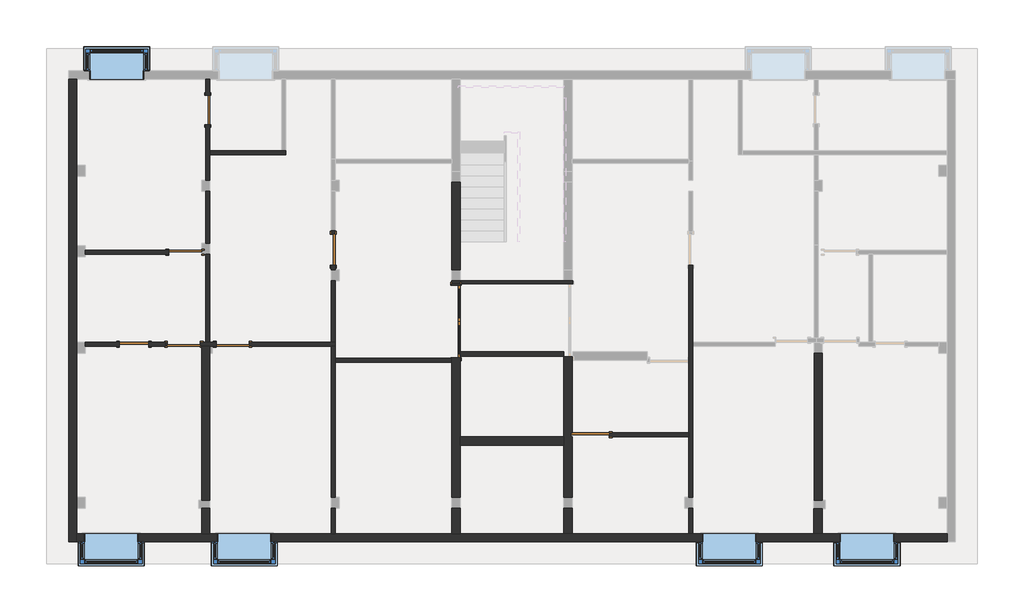
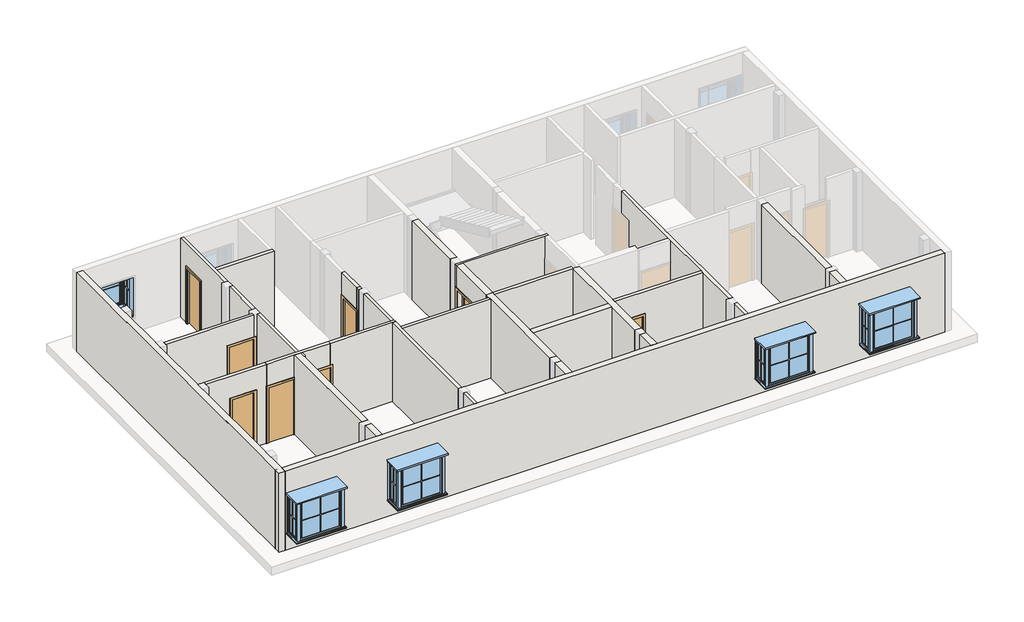
# One storey, part 1 of 3: 33 walls, 8 doors, 5 windows.
"""IFC4 building model written with IfcOpenShell, lengths in millimetres."""

from ifc_helpers import new_model, si_unit, frame, origin, place, context, project, spatial, polyline, outline, extrude, faceted_brep, transform, mapped, element, save
from components import door_77e2dd85, m_door_single_panel_05506f71, door_07b5d71c, door_4c0a2014, door_82def9da, m_door_single_panel_3_x7_f8176753, m_door_single_panel_3_x7_ebb67e73, window_19bbd869

model = new_model("IFC4")

# Units and contexts
model_context = context("Model", 3, world=origin())
ifc_project = project(units=[si_unit("LENGTHUNIT", "METRE", prefix="MILLI")], contexts=[model_context])

# Site, building, storey
site = spatial("IfcSite", under=ifc_project)
building = spatial("IfcBuilding", under=site)
storey = spatial("IfcBuildingStorey", under=building, Elevation=12801.6)

# Doors
placement = place(None, origin())
door_shape = door_77e2dd85(model_context)
element("IfcDoor", 1, ObjectType="M_Door-Double-Glass : 6'7\"X7'", at=placement, inside=storey, context=model_context, shape_type="MappedRepresentation", body=[
    mapped(door_shape, transform((-1965.4800498, 1154.8067742, 12801.6), x_axis=(0.0, -1.0, 0.0), y_axis=(1.0, 0.0, 0.0), z_axis=(0.0, 0.0, 1.0))),
])
m_door_single_panel_shape = m_door_single_panel_05506f71(model_context)
element("IfcDoor", 2, ObjectType="M_Door-Single-Panel", at=placement, inside=storey, context=model_context, shape_type="MappedRepresentation", body=[
    mapped(m_door_single_panel_shape, transform((1745.3012085, -1975.7432663, 12801.6), x_axis=(-1.0, 0.0, 0.0), y_axis=(0.0, -1.0, 0.0), z_axis=(0.0, 0.0, 1.0))),
])
door_2_shape = door_07b5d71c(model_context)
element("IfcDoor", 3, ObjectType="M_Door-Single-Panel : 2'10\"X7' 2", at=placement, inside=storey, context=model_context, shape_type="MappedRepresentation", body=[
    mapped(door_2_shape, transform((-5360.3487995, 3142.9626891, 12801.6), x_axis=(0.0, -1.0, 0.0), y_axis=(1.0, 0.0, 0.0), z_axis=(0.0, 0.0, 1.0))),
])
door_3_shape = door_4c0a2014(model_context)
element("IfcDoor", 4, ObjectType="M_Door-Single-Panel : 2'8\"X7'", at=placement, inside=storey, context=model_context, shape_type="MappedRepresentation", body=[
    mapped(door_3_shape, transform((-10873.4462614, 526.1567334, 12801.6), x_axis=(1.0, 0.0, 0.0), y_axis=(0.0, 1.0, 0.0), z_axis=(0.0, 0.0, 1.0))),
])
door_4_shape = door_82def9da(model_context)
element("IfcDoor", 5, ObjectType="M_Door-Single-Panel : 2'8\"X7'", at=placement, inside=storey, context=model_context, shape_type="MappedRepresentation", body=[
    mapped(door_4_shape, transform((-8827.4487992, 7008.6751452, 12801.6), x_axis=(0.0, 1.0, 0.0), y_axis=(-1.0, 0.0, 0.0), z_axis=(0.0, 0.0, 1.0))),
])
m_door_single_panel_3_x7_shape = m_door_single_panel_3_x7_f8176753(model_context)
element("IfcDoor", 6, ObjectType="M_Door-Single-Panel : 3'X7'", at=placement, inside=storey, context=model_context, shape_type="MappedRepresentation", body=[
    mapped(m_door_single_panel_3_x7_shape, transform((-9456.0987989, 3078.8567332, 12801.6), x_axis=(1.0, 0.0, 0.0), y_axis=(0.0, 1.0, 0.0), z_axis=(0.0, 0.0, 1.0))),
])
element("IfcDoor", 7, ObjectType="M_Door-Single-Panel : 3'X7'", at=placement, inside=storey, context=model_context, shape_type="MappedRepresentation", body=[
    mapped(m_door_single_panel_3_x7_shape, transform((-8144.8381465, 526.1567334, 12801.6), x_axis=(-1.0, 0.0, 0.0), y_axis=(0.0, -1.0, 0.0), z_axis=(0.0, 0.0, 1.0))),
])
m_door_single_panel_3_x7_2_shape = m_door_single_panel_3_x7_ebb67e73(model_context)
element("IfcDoor", 8, ObjectType="M_Door-Single-Panel : 3'X7'", at=placement, inside=storey, context=model_context, shape_type="MappedRepresentation", body=[
    mapped(m_door_single_panel_3_x7_2_shape, transform((-9494.1987992, 526.1567334, 12801.6), x_axis=(1.0, 0.0, 0.0), y_axis=(0.0, 1.0, 0.0), z_axis=(0.0, 0.0, 1.0))),
])

# Walls
element("IfcWall", 9, ObjectType="3.5\"", at=placement, inside=storey, context=model_context, shape_type="Brep", body=[
    faceted_brep([(-2077.3987998, 2196.2067742, 12801.6), (-1848.7987998, 2196.2067742, 12801.6), (1158.0082462, 2196.2067742, 12801.6), (1272.3082462, 2196.2067742, 12801.6), (1272.3082462, 2196.2067742, 15849.6), (1158.0082462, 2196.2067742, 15849.6), (-1848.7987998, 2196.2067742, 15849.6), (-2077.3987998, 2196.2067742, 15849.6), (-2077.3987998, 2285.1067742, 12801.6), (-2077.3987998, 2285.1067742, 15849.6), (-2074.1417538, 2285.1067742, 15849.6), (-1845.5417538, 2285.1067742, 15849.6), (1024.6582462, 2285.1067742, 15849.6), (1253.2582462, 2285.1067742, 15849.6), (1272.3082462, 2285.1067742, 15849.6), (1272.3082462, 2285.1067742, 12801.6), (1253.2582462, 2285.1067742, 12801.6), (1024.6582462, 2285.1067742, 12801.6), (-1845.5417538, 2285.1067742, 12801.6), (-2074.1417538, 2285.1067742, 12801.6)], [[[0, 1, 2, 3, 4, 5, 6, 7]], [[8, 9, 10, 11, 12, 13, 14, 15, 16, 17, 18, 19]], [[3, 2, 1, 0, 8, 19, 18, 17, 16, 15]], [[7, 6, 5, 4, 14, 13, 12, 11, 10, 9]], [[4, 3, 15, 14]], [[0, 7, 9, 8]]]),
])
element("IfcWall", 10, ObjectType="4.5\"", at=placement, inside=storey, context=model_context, shape_type="SweptSolid", body=[
    extrude(outline(polyline([(2711.1626891, 15849.6), (3671.8272228, 15849.6), (3671.8272228, 12801.6), (3574.7626891, 12801.6), (3574.7626891, 14935.2), (2711.1626891, 14935.2), (2711.1626891, 15849.6)])), frame((-5417.4987995, 0.0, 0.0), z_axis=(1.0, 0.0, 0.0), x_axis=(0.0, 1.0, 0.0)), (0.0, 0.0, 1.0), 114.3),
])
element("IfcWall", 11, ObjectType="4.5\"", at=placement, inside=storey, context=model_context, shape_type="Brep", body=[
    faceted_brep([(-7690.1644155, 469.0067334, 15849.6), (-8713.148796, 469.0067334, 15849.6), (-8771.750543, 469.0067334, 15849.6), (-9000.350543, 469.0067334, 15849.6), (-10009.8462614, 469.0067334, 15849.6), (-10009.8462614, 469.0067334, 12801.6), (-9951.3987992, 469.0067334, 12801.6), (-9951.3987992, 469.0067334, 14935.2), (-9036.9987992, 469.0067334, 14935.2), (-9036.9987992, 469.0067334, 12801.6), (-9000.350543, 469.0067334, 12801.6), (-8771.750543, 469.0067334, 12801.6), (-8713.148796, 469.0067334, 12801.6), (-8602.0381465, 469.0067334, 12801.6), (-8602.0381465, 469.0067334, 14935.2), (-7690.1644155, 469.0067334, 14935.2), (-10009.8462614, 583.3067334, 15849.6), (-7690.1644155, 583.3067334, 15849.6), (-7690.1644155, 583.3067334, 14935.2), (-8602.0381465, 583.3067334, 14935.2), (-8602.0381465, 583.3067334, 12801.6), (-9036.9987992, 583.3067334, 12801.6), (-9036.9987992, 583.3067334, 14935.2), (-9951.3987992, 583.3067334, 14935.2), (-9951.3987992, 583.3067334, 12801.6), (-10009.8462614, 583.3067334, 12801.6)], [[[0, 1, 2, 3, 4, 5, 6, 7, 8, 9, 10, 11, 12, 13, 14, 15]], [[16, 17, 18, 19, 20, 21, 22, 23, 24, 25]], [[5, 25, 24, 6]], [[9, 21, 20, 13, 12, 11, 10]], [[17, 0, 15, 18]], [[4, 3, 2, 1, 0, 17, 16]], [[5, 4, 16, 25]], [[8, 22, 21, 9]], [[7, 23, 22, 8]], [[23, 7, 6, 24]], [[19, 14, 13, 20]], [[14, 19, 18, 15]]]),
])
element("IfcWall", 12, ObjectType="4.5\"", at=placement, inside=storey, context=model_context, shape_type="SweptSolid", body=[
    extrude(outline(polyline([(15849.6, 4475.8012082), (15849.6, 1250.0012085), (14935.2, 1250.0012085), (14935.2, 2278.7012085), (12801.6, 2278.7012085), (12801.6, 4475.8012082), (15849.6, 4475.8012082)])), frame((0.0, -2032.8932663, 0.0), z_axis=(0.0, 1.0, 0.0), x_axis=(0.0, 0.0, 1.0)), (0.0, 0.0, 1.0), 114.3),
])
element("IfcWall", 13, ObjectType="4.5\"", at=placement, inside=storey, context=model_context, shape_type="Brep", body=[
    faceted_brep([(-1848.7987998, 202.3067742, 12801.6), (1021.4012085, 202.3067742, 12801.6), (1021.4012085, 202.3067742, 15849.6), (-1848.7987998, 202.3067742, 15849.6), (-1848.7987998, 316.6067742, 12801.6), (-1848.7987998, 316.6067742, 14935.2), (-1848.7987998, 316.6067742, 15849.6), (1021.4012085, 316.6067742, 15849.6), (1021.4012085, 316.6067742, 12801.6)], [[[0, 1, 2, 3]], [[4, 5, 6, 7, 8]], [[1, 0, 4, 8]], [[2, 1, 8, 7]], [[3, 2, 7, 6]], [[0, 3, 6, 5, 4]]]),
])
element("IfcWall", 14, ObjectType="4.5\"", at=placement, inside=storey, context=model_context, shape_type="Brep", body=[
    faceted_brep([(-5417.4987995, 469.0067334, 12801.6), (-5417.4987995, -3709.2932193, 12801.6), (-5417.4987995, -3709.2932193, 15849.6), (-5417.4987995, 469.0067334, 15849.6), (-5303.1987995, 469.0067334, 12801.6), (-5303.1987995, 469.0067334, 15849.6), (-5303.1987995, 148.1078621, 15849.6), (-5303.1987995, 33.8078621, 15849.6), (-5303.1987995, -3709.2932193, 15849.6), (-5303.1987995, -3709.2932193, 12801.6), (-5303.1987995, 33.8078621, 12801.6), (-5303.1987995, 148.1078621, 12801.6)], [[[0, 1, 2, 3]], [[4, 5, 6, 7, 8, 9, 10, 11]], [[1, 0, 4, 11, 10, 9]], [[2, 1, 9, 8]], [[3, 2, 8, 7, 6, 5]], [[0, 3, 5, 4]]]),
])
element("IfcWall", 15, ObjectType="4.5\"", at=placement, inside=storey, context=model_context, shape_type="SweptSolid", body=[
    extrude(outline(polyline([(-5417.4987963, -4712.5932661), (-5417.4987963, -4014.0932193), (-5303.1987963, -4014.0932193), (-5303.1987963, -4712.5932661), (-5417.4987963, -4712.5932661)])), frame((0.0, 0.0, 12801.6), z_axis=(0.0, 0.0, 1.0), x_axis=(1.0, 0.0, 0.0)), (0.0, 0.0, 1.0), 3048.0),
])
element("IfcWall", 16, ObjectType="4.5\"", at=placement, inside=storey, context=model_context, shape_type="SweptSolid", body=[
    extrude(outline(polyline([(4475.8012082, -4712.5932661), (4475.8012082, -4014.0932193), (4590.1012082, -4014.0932193), (4590.1012082, -4712.5932661), (4475.8012082, -4712.5932661)])), frame((0.0, 0.0, 12801.6), z_axis=(0.0, 0.0, 1.0), x_axis=(1.0, 0.0, 0.0)), (0.0, 0.0, 1.0), 3048.0),
])
element("IfcWall", 17, ObjectType="4.5\" 2", at=placement, inside=storey, context=model_context, shape_type="SweptSolid", body=[
    extrude(outline(polyline([(15849.6, -8998.8987989), (15849.6, -12224.6987989), (12801.6, -12224.6987989), (12801.6, -9913.2987989), (14935.2, -9913.2987989), (14935.2, -8998.8987989), (15849.6, -8998.8987989)])), frame((0.0, 3021.7067332, 0.0), z_axis=(0.0, 1.0, 0.0), x_axis=(0.0, 0.0, 1.0)), (0.0, 0.0, 1.0), 114.3),
])
element("IfcWall", 18, ObjectType="4.5\" 2", at=placement, inside=storey, context=model_context, shape_type="SweptSolid", body=[
    extrude(outline(polyline([(-8770.2987992, 4761.606733), (-8770.2987992, 3326.5067332), (-8884.5987992, 3326.5067332), (-8884.5987992, 4761.606733), (-8770.2987992, 4761.606733)])), frame((0.0, 0.0, 12801.6), z_axis=(0.0, 0.0, 1.0), x_axis=(1.0, 0.0, 0.0)), (0.0, 0.0, 1.0), 3048.0),
])
element("IfcWall", 19, ObjectType="4.5\" 2", at=placement, inside=storey, context=model_context, shape_type="Brep", body=[
    faceted_brep([(-8770.2987992, 7415.0751452, 14935.2), (-8770.2987992, 7415.0751452, 12801.6), (-8770.2987992, 7860.4067329, 12801.6), (-8770.2987992, 7860.4067329, 15849.6), (-8770.2987992, 5879.2067329, 15849.6), (-8770.2987992, 5764.9067329, 15849.6), (-8770.2987992, 5066.406733, 15849.6), (-8770.2987992, 5066.406733, 12801.6), (-8770.2987992, 5764.9067329, 12801.6), (-8770.2987992, 5879.2067329, 12801.6), (-8770.2987992, 6602.2751452, 12801.6), (-8770.2987992, 6602.2751452, 14935.2), (-8884.5987992, 7860.4067329, 12801.6), (-8884.5987992, 7415.0751452, 12801.6), (-8884.5987992, 7415.0751452, 14935.2), (-8884.5987992, 6602.2751452, 14935.2), (-8884.5987992, 6602.2751452, 12801.6), (-8884.5987992, 5066.406733, 12801.6), (-8884.5987992, 5066.406733, 15849.6), (-8884.5987992, 7860.4067329, 15849.6)], [[[0, 1, 2, 3, 4, 5, 6, 7, 8, 9, 10, 11]], [[12, 13, 14, 15, 16, 17, 18, 19]], [[2, 1, 13, 12]], [[10, 9, 8, 7, 17, 16]], [[6, 5, 4, 3, 19, 18]], [[7, 6, 18, 17]], [[14, 13, 1, 0]], [[15, 14, 0, 11]], [[16, 15, 11, 10]], [[3, 2, 12, 19]]]),
])
element("IfcWall", 20, ObjectType="4.5\" 2", at=placement, inside=storey, context=model_context, shape_type="Brep", body=[
    faceted_brep([(-8770.2987992, 5764.9067329, 12801.6), (-6674.7987994, 5764.9067329, 12801.6), (-6674.7987994, 5764.9067329, 15849.6), (-8770.2987992, 5764.9067329, 15849.6), (-8770.2987992, 5879.2067329, 12801.6), (-8770.2987992, 5879.2067329, 15849.6), (-6789.0987994, 5879.2067329, 15849.6), (-6674.7987994, 5879.2067329, 15849.6), (-6674.7987994, 5879.2067329, 12801.6), (-6789.0987994, 5879.2067329, 12801.6)], [[[0, 1, 2, 3]], [[4, 5, 6, 7, 8, 9]], [[1, 0, 4, 9, 8]], [[3, 2, 7, 6, 5]], [[0, 3, 5, 4]], [[2, 1, 8, 7]]]),
])
element("IfcWall", 21, ObjectType="4.5\" 2", at=placement, inside=storey, context=model_context, shape_type="SweptSolid", body=[
    extrude(outline(polyline([(14935.2, -10467.0462614), (12801.6, -10467.0462614), (12801.6, -10009.8462614), (15849.6, -10009.8462614), (15849.6, -12224.6987989), (12801.6, -12224.6987989), (12801.6, -11279.8462614), (14935.2, -11279.8462614), (14935.2, -10467.0462614)])), frame((0.0, 469.0067334, 0.0), z_axis=(0.0, 1.0, 0.0), x_axis=(0.0, 0.0, 1.0)), (0.0, 0.0, 1.0), 114.3),
])
element("IfcWall", 22, ObjectType="4.5\" 2", at=placement, inside=storey, context=model_context, shape_type="SweptSolid", body=[
    extrude(outline(polyline([(-8770.298796, 3021.7067332), (-8770.298796, 583.3067804), (-8884.598796, 583.3067804), (-8884.598796, 3021.7067332), (-8770.298796, 3021.7067332)])), frame((0.0, 0.0, 12801.6), z_axis=(0.0, 0.0, 1.0), x_axis=(1.0, 0.0, 0.0)), (0.0, 0.0, 1.0), 3048.0),
])
element("IfcWall", 23, ObjectType="4.5\" 2", at=placement, inside=storey, context=model_context, shape_type="Brep", body=[
    faceted_brep([(-5303.1987995, 469.0067334, 15849.6), (-5417.4987995, 469.0067334, 15849.6), (-7690.1644155, 469.0067334, 15849.6), (-7690.1644155, 469.0067334, 14935.2), (-7687.6381465, 469.0067334, 14935.2), (-7687.6381465, 469.0067334, 12801.6), (-5417.4987995, 469.0067334, 12801.6), (-5303.1987995, 469.0067334, 12801.6), (-7690.1644155, 583.3067334, 15849.6), (-5417.4987995, 583.3067334, 15849.6), (-5303.1987995, 583.3067334, 15849.6), (-5303.1987995, 583.3067334, 12801.6), (-5417.4987995, 583.3067334, 12801.6), (-7687.6381465, 583.3067334, 12801.6), (-7687.6381465, 583.3067334, 14935.2), (-7690.1644155, 583.3067334, 14935.2)], [[[0, 1, 2, 3, 4, 5, 6, 7]], [[8, 9, 10, 11, 12, 13, 14, 15]], [[11, 7, 6, 5, 13, 12]], [[2, 1, 0, 10, 9, 8]], [[2, 8, 15, 3]], [[0, 7, 11, 10]], [[14, 4, 3, 15]], [[4, 14, 13, 5]]]),
])
element("IfcWall", 24, ObjectType="4.5\" 2", at=placement, inside=storey, context=model_context, shape_type="SweptSolid", body=[
    extrude(outline(polyline([(-5303.1987995, 2285.1067802), (-5303.1987995, 583.3067334), (-5417.4987995, 583.3067334), (-5417.4987995, 2285.1067802), (-5303.1987995, 2285.1067802)])), frame((0.0, 0.0, 12801.6), z_axis=(0.0, 0.0, 1.0), x_axis=(1.0, 0.0, 0.0)), (0.0, 0.0, 1.0), 3048.0),
])
element("IfcWall", 25, ObjectType="4.5\" 2", at=placement, inside=storey, context=model_context, shape_type="Brep", body=[
    faceted_brep([(-5303.1987995, 2589.9067802, 12801.6), (-5303.1987995, 2711.1626891, 12801.6), (-5303.1987995, 2711.1626891, 14935.2), (-5303.1987995, 2711.1626891, 15849.6), (-5303.1987995, 2589.9067802, 15849.6), (-5417.4987995, 2589.9067802, 12801.6), (-5417.4987995, 2589.9067802, 15849.6), (-5417.4987995, 2711.1626891, 15849.6), (-5417.4987995, 2711.1626891, 14935.2), (-5417.4987995, 2711.1626891, 12801.6)], [[[0, 1, 2, 3, 4]], [[5, 6, 7, 8, 9]], [[1, 0, 5, 9]], [[3, 2, 1, 9, 8, 7]], [[4, 3, 7, 6]], [[0, 4, 6, 5]]]),
])
element("IfcWall", 26, ObjectType="4.5\" 2", at=placement, inside=storey, context=model_context, shape_type="Brep", body=[
    faceted_brep([(4475.8012082, -3709.2932193, 12801.6), (4475.8012082, -3709.2932193, 15849.6), (4475.8012082, -2032.8932663, 15849.6), (4475.8012082, -1918.5932663, 15849.6), (4475.8012082, 33.8078621, 15849.6), (4475.8012082, 148.1078621, 15849.6), (4475.8012082, 3132.0737955, 15849.6), (4475.8012082, 3132.0737955, 14935.2), (4475.8012082, 2711.1626891, 14935.2), (4475.8012082, 2711.1626891, 12801.6), (4475.8012082, 148.1078621, 12801.6), (4475.8012082, 33.8078621, 12801.6), (4475.8012082, -1918.5932663, 12801.6), (4475.8012082, -2032.8932663, 12801.6), (4590.1012082, -3709.2932193, 15849.6), (4590.1012082, -3709.2932193, 12801.6), (4590.1012082, 469.0067334, 12801.6), (4590.1012082, 583.3067334, 12801.6), (4590.1012082, 2711.1626891, 12801.6), (4590.1012082, 2711.1626891, 14935.2), (4590.1012082, 3132.0737955, 14935.2), (4590.1012082, 3132.0737955, 15849.6), (4590.1012082, 583.3067334, 15849.6), (4590.1012082, 469.0067334, 15849.6)], [[[0, 1, 2, 3, 4, 5, 6, 7, 8, 9, 10, 11, 12, 13]], [[14, 15, 16, 17, 18, 19, 20, 21, 22, 23]], [[15, 0, 13, 12, 11, 10, 9, 18, 17, 16]], [[1, 0, 15, 14]], [[6, 5, 4, 3, 2, 1, 14, 23, 22, 21]], [[6, 21, 20, 7]], [[8, 19, 18, 9]], [[19, 8, 7, 20]]]),
])
element("IfcWall", 27, ObjectType="4.5\" 2", at=placement, inside=storey, context=model_context, shape_type="SweptSolid", body=[
    extrude(outline(polyline([(-2077.3987998, 33.8078621), (-5303.1987995, 33.8078621), (-5303.1987995, 148.1078621), (-2077.3987998, 148.1078621), (-2077.3987998, 33.8078621)])), frame((0.0, 0.0, 12801.6), z_axis=(0.0, 0.0, 1.0), x_axis=(1.0, 0.0, 0.0)), (0.0, 0.0, 1.0), 3048.0),
])
element("IfcWall", 28, ObjectType="9\"", at=placement, inside=storey, context=model_context, shape_type="Brep", body=[
    faceted_brep([(-12453.2987957, -4941.1932661, 12801.6), (-12453.2987957, -4712.5932661, 12801.6), (-12453.2987957, -4014.0932671, 12801.6), (-12453.2987957, -3709.2932671, 12801.6), (-12453.2987957, 278.5067334, 12801.6), (-12453.2987957, 583.3067334, 12801.6), (-12453.2987957, 2951.8567332, 12801.6), (-12453.2987957, 3256.6567332, 12801.6), (-12453.2987957, 5174.3567339, 12801.6), (-12453.2987957, 5479.1567339, 12801.6), (-12453.2987957, 7860.4067329, 12801.6), (-12453.2987957, 7860.4067329, 15849.6), (-12453.2987957, 5479.1567339, 15849.6), (-12453.2987957, 5174.3567339, 15849.6), (-12453.2987957, 3256.6567332, 15849.6), (-12453.2987957, 2951.8567332, 15849.6), (-12453.2987957, 583.3067334, 15849.6), (-12453.2987957, 278.5067334, 15849.6), (-12453.2987957, -3709.2932671, 15849.6), (-12453.2987957, -4014.0932671, 15849.6), (-12453.2987957, -4712.5932661, 15849.6), (-12453.2987957, -4941.1932661, 15849.6), (-12681.8987957, -4941.1932661, 12801.6), (-12681.8987957, -4941.1932661, 15849.6), (-12681.8987957, 7860.4067329, 15849.6), (-12681.8987957, 7860.4067329, 12801.6)], [[[0, 1, 2, 3, 4, 5, 6, 7, 8, 9, 10, 11, 12, 13, 14, 15, 16, 17, 18, 19, 20, 21]], [[22, 23, 24, 25]], [[10, 9, 8, 7, 6, 5, 4, 3, 2, 1, 0, 22, 25]], [[21, 20, 19, 18, 17, 16, 15, 14, 13, 12, 11, 24, 23]], [[11, 10, 25, 24]], [[0, 21, 23, 22]]]),
])
element("IfcWall", 29, ObjectType="9\"", at=placement, inside=storey, context=model_context, shape_type="Brep", body=[
    faceted_brep([(-12453.2987957, -4712.5932661, 12801.6), (-12453.2987957, -4014.0932671, 12801.6), (-12453.2987957, -3709.2932671, 12801.6), (-12453.2987957, 278.5067334, 12801.6), (-12453.2987957, 583.3067334, 12801.6), (-12453.2987957, 2951.8567332, 12801.6), (-12453.2987957, 3256.6567332, 12801.6), (-12453.2987957, 5174.3567339, 12801.6), (-12453.2987957, 5479.1567339, 12801.6), (-12453.2987957, 7860.4067329, 12801.6), (-12453.2987957, 7860.4067329, 15849.6), (-12453.2987957, 5479.1567339, 15849.6), (-12453.2987957, 5174.3567339, 15849.6), (-12453.2987957, 3256.6567332, 15849.6), (-12453.2987957, 2951.8567332, 15849.6), (-12453.2987957, 583.3067334, 15849.6), (-12453.2987957, 278.5067334, 15849.6), (-12453.2987957, -3709.2932671, 15849.6), (-12453.2987957, -4014.0932671, 15849.6), (-12453.2987957, -4712.5932661, 15849.6), (-12681.8987957, -4712.5932661, 12801.6), (-12681.8987957, -4712.5932661, 15849.6), (-12681.8987957, 7860.4067329, 15849.6), (-12681.8987957, 7860.4067329, 12801.6)], [[[0, 1, 2, 3, 4, 5, 6, 7, 8, 9, 10, 11, 12, 13, 14, 15, 16, 17, 18, 19]], [[20, 21, 22, 23]], [[9, 8, 7, 6, 5, 4, 3, 2, 1, 0, 20, 23]], [[19, 18, 17, 16, 15, 14, 13, 12, 11, 10, 22, 21]], [[10, 9, 23, 22]], [[0, 19, 21, 20]]]),
])
element("IfcWall", 30, ObjectType="9\"", at=placement, inside=storey, context=model_context, shape_type="Brep", body=[
    faceted_brep([(-9000.350543, 469.0067334, 12801.6), (-9000.350543, -3785.4932196, 12801.6), (-9000.350543, -3785.4932196, 15849.6), (-9000.350543, 469.0067334, 15849.6), (-8771.750543, 469.0067334, 12801.6), (-8771.750543, 469.0067334, 15849.6), (-8771.750543, 278.5067334, 15849.6), (-8771.750543, -3785.4932196, 15849.6), (-8771.750543, -3785.4932196, 12801.6), (-8771.750543, 278.5067334, 12801.6)], [[[0, 1, 2, 3]], [[4, 5, 6, 7, 8, 9]], [[1, 0, 4, 9, 8]], [[2, 1, 8, 7]], [[3, 2, 7, 6, 5]], [[0, 3, 5, 4]]]),
])
element("IfcWall", 31, ObjectType="9\"", at=placement, inside=storey, context=model_context, shape_type="Brep", body=[
    faceted_brep([(-2077.3987998, -3709.2932663, 12801.6), (-2077.3987998, -3709.2932663, 15849.6), (-2077.3987998, 33.8078621, 15849.6), (-2077.3987998, 148.1078621, 15849.6), (-2077.3987998, 316.6067742, 15849.6), (-2077.3987998, 316.6067742, 14935.2), (-2077.3987998, 151.5067742, 14935.2), (-2077.3987998, 151.5067742, 12801.6), (-2077.3987998, 148.1078621, 12801.6), (-2077.3987998, 33.8078621, 12801.6), (-1848.7987998, -3709.2932663, 15849.6), (-1848.7987998, -3709.2932663, 12801.6), (-1848.7987998, -2261.4932663, 12801.6), (-1848.7987998, -2032.8932663, 12801.6), (-1848.7987998, 151.5067742, 12801.6), (-1848.7987998, 151.5067742, 14935.2), (-1848.7987998, 316.6067742, 14935.2), (-1848.7987998, 316.6067742, 15849.6), (-1848.7987998, 202.3067742, 15849.6), (-1848.7987998, -2032.8932663, 15849.6), (-1848.7987998, -2261.4932663, 15849.6)], [[[0, 1, 2, 3, 4, 5, 6, 7, 8, 9]], [[10, 11, 12, 13, 14, 15, 16, 17, 18, 19, 20]], [[11, 0, 9, 8, 7, 14, 13, 12]], [[1, 0, 11, 10]], [[4, 3, 2, 1, 10, 20, 19, 18, 17]], [[4, 17, 16, 5]], [[6, 15, 14, 7]], [[15, 6, 5, 16]]]),
])
element("IfcWall", 32, ObjectType="9\"", at=placement, inside=storey, context=model_context, shape_type="SweptSolid", body=[
    extrude(outline(polyline([(1021.4012085, -2261.4932663), (-1848.7987998, -2261.4932663), (-1848.7987998, -2032.8932663), (1021.4012085, -2032.8932663), (1021.4012085, -2261.4932663)])), frame((0.0, 0.0, 12801.6), z_axis=(0.0, 0.0, 1.0), x_axis=(1.0, 0.0, 0.0)), (0.0, 0.0, 1.0), 3048.0),
])
element("IfcWall", 33, ObjectType="9\"", at=placement, inside=storey, context=model_context, shape_type="Brep", body=[
    faceted_brep([(1021.4012085, -3709.2932193, 12801.6), (1021.4012085, -3709.2932193, 15849.6), (1021.4012085, -2261.4932663, 15849.6), (1021.4012085, -2032.8932663, 15849.6), (1021.4012085, 205.2578621, 15849.6), (1021.4012085, 205.2578621, 14935.2), (1021.4012085, 180.0817656, 14935.2), (1021.4012085, 180.0817656, 12801.6), (1021.4012085, -2032.8932663, 12801.6), (1021.4012085, -2261.4932663, 12801.6), (1250.0012085, -3709.2932193, 15849.6), (1250.0012085, -3709.2932193, 12801.6), (1250.0012085, -2032.8932663, 12801.6), (1250.0012085, -2032.8932663, 14935.2), (1250.0012085, -1918.5932663, 14935.2), (1250.0012085, -1918.5932663, 12801.6), (1250.0012085, 90.9578621, 12801.6), (1250.0012085, 180.0817656, 12801.6), (1250.0012085, 180.0817656, 14935.2), (1250.0012085, 205.2578621, 14935.2), (1250.0012085, 205.2578621, 15849.6), (1250.0012085, 90.9578621, 15849.6), (1250.0012085, -1918.5932663, 15849.6), (1250.0012085, -2032.8932663, 15849.6), (1211.9012085, -1918.5932663, 12801.6), (1211.9012085, -2032.8932663, 12801.6), (1158.0082462, 205.2578621, 15849.6), (1158.0082462, 205.2578621, 14935.2), (1211.9012085, -1918.5932663, 14935.2), (1211.9012085, -2032.8932663, 14935.2)], [[[0, 1, 2, 3, 4, 5, 6, 7, 8, 9]], [[10, 11, 12, 13, 14, 15, 16, 17, 18, 19, 20, 21, 22, 23]], [[11, 0, 9, 8, 7, 17, 16, 15, 24, 25, 12]], [[1, 0, 11, 10]], [[4, 3, 2, 1, 10, 23, 22, 21, 20, 26]], [[4, 26, 20, 19, 27, 5]], [[28, 24, 15, 14]], [[25, 29, 13, 12]], [[24, 28, 29, 25]], [[29, 28, 14, 13]], [[18, 6, 5, 27, 19]], [[6, 18, 17, 7]]]),
])
element("IfcWall", 34, ObjectType="9\"", at=placement, inside=storey, context=model_context, shape_type="SweptSolid", body=[
    extrude(outline(polyline([(-2074.1417538, 2589.906774), (-2074.1417538, 5015.606774), (-1845.5417538, 5015.606774), (-1845.5417538, 2589.906774), (-2074.1417538, 2589.906774)])), frame((0.0, 0.0, 12801.6), z_axis=(0.0, 0.0, 1.0), x_axis=(1.0, 0.0, 0.0)), (0.0, 0.0, 1.0), 3048.0),
])
element("IfcWall", 35, ObjectType="9\"", at=placement, inside=storey, context=model_context, shape_type="SweptSolid", body=[
    extrude(outline(polyline([(7942.9012047, -3785.4932666), (7942.9012047, 278.5067334), (8171.5012047, 278.5067334), (8171.5012047, -3785.4932666), (7942.9012047, -3785.4932666)])), frame((0.0, 0.0, 12801.6), z_axis=(0.0, 0.0, 1.0), x_axis=(1.0, 0.0, 0.0)), (0.0, 0.0, 1.0), 3048.0),
])
element("IfcWall", 36, ObjectType="9\"", at=placement, inside=storey, context=model_context, shape_type="SweptSolid", body=[
    extrude(outline(polyline([(-2077.3987998, -4712.5932661), (-2077.3987998, -4014.0932663), (-1848.7987998, -4014.0932663), (-1848.7987998, -4712.5932661), (-2077.3987998, -4712.5932661)])), frame((0.0, 0.0, 12801.6), z_axis=(0.0, 0.0, 1.0), x_axis=(1.0, 0.0, 0.0)), (0.0, 0.0, 1.0), 3048.0),
])
element("IfcWall", 37, ObjectType="9\"", at=placement, inside=storey, context=model_context, shape_type="SweptSolid", body=[
    extrude(outline(polyline([(1021.4012085, -4712.5932661), (1021.4012085, -4014.0932193), (1250.0012085, -4014.0932193), (1250.0012085, -4712.5932661), (1021.4012085, -4712.5932661)])), frame((0.0, 0.0, 12801.6), z_axis=(0.0, 0.0, 1.0), x_axis=(1.0, 0.0, 0.0)), (0.0, 0.0, 1.0), 3048.0),
])
element("IfcWall", 38, ObjectType="9\"", at=placement, inside=storey, context=model_context, shape_type="SweptSolid", body=[
    extrude(outline(polyline([(7941.7646942, -4712.5932661), (7941.7646942, -4015.9914801), (8170.3646942, -4015.9914801), (8170.3646942, -4712.5932661), (7941.7646942, -4712.5932661)])), frame((0.0, 0.0, 12801.6), z_axis=(0.0, 0.0, 1.0), x_axis=(1.0, 0.0, 0.0)), (0.0, 0.0, 1.0), 3048.0),
])
element("IfcWall", 39, ObjectType="9\"", at=placement, inside=storey, context=model_context, shape_type="SweptSolid", body=[
    extrude(outline(polyline([(-9000.350543, -4712.5932661), (-9000.350543, -4014.0932196), (-8771.750543, -4014.0932196), (-8771.750543, -4712.5932661), (-9000.350543, -4712.5932661)])), frame((0.0, 0.0, 12801.6), z_axis=(0.0, 0.0, 1.0), x_axis=(1.0, 0.0, 0.0)), (0.0, 0.0, 1.0), 3048.0),
])
element("IfcWall", 40, ObjectType="9\"", at=placement, inside=storey, context=model_context, shape_type="SweptSolid", body=[
    extrude(outline(polyline([(316.6067742, 15849.6), (2196.2067742, 15849.6), (2196.2067742, 12801.6), (2158.1067742, 12801.6), (2158.1067742, 14935.2), (316.6067742, 14935.2), (316.6067742, 15849.6)])), frame((-2077.3987998, 0.0, 0.0), z_axis=(1.0, 0.0, 0.0), x_axis=(0.0, 1.0, 0.0)), (0.0, 0.0, 1.0), 228.6),
])
element("IfcWall", 41, ObjectType="9\" 2", at=placement, inside=storey, context=model_context, shape_type="Brep", body=[
    faceted_brep([(-12453.2987957, -4941.1932661, 12801.6), (11625.9012075, -4941.1932662, 12801.6), (11625.9012075, -4941.1932662, 15849.6), (-12453.2987957, -4941.1932661, 15849.6), (8658.6146942, -4941.1932661, 14952.4), (10158.6146942, -4941.1932661, 14952.4), (10158.6146942, -4941.1932661, 13401.6), (8658.6146942, -4941.1932661, 13401.6), (4849.7512082, -4941.1932661, 14952.4), (6349.7512082, -4941.1932661, 14952.4), (6349.7512082, -4941.1932661, 13401.6), (4849.7512082, -4941.1932661, 13401.6), (-8569.250543, -4941.1932661, 14952.4), (-7069.250543, -4941.1932661, 14952.4), (-7069.250543, -4941.1932661, 13401.6), (-8569.250543, -4941.1932661, 13401.6), (-12250.7987957, -4941.1932661, 14952.4), (-10750.7987957, -4941.1932661, 14952.4), (-10750.7987957, -4941.1932661, 13401.6), (-12250.7987957, -4941.1932661, 13401.6), (-12453.2987957, -4712.5932661, 12801.6), (-12453.2987957, -4712.5932661, 15849.6), (-9000.350543, -4712.5932661, 15849.6), (-8771.750543, -4712.5932661, 15849.6), (-5417.4987963, -4712.5932661, 15849.6), (-5303.1987963, -4712.5932661, 15849.6), (-2077.3987998, -4712.5932661, 15849.6), (-1848.7987998, -4712.5932661, 15849.6), (1021.4012085, -4712.5932661, 15849.6), (1250.0012085, -4712.5932661, 15849.6), (4475.8012082, -4712.5932661, 15849.6), (4590.1012082, -4712.5932661, 15849.6), (7941.7646942, -4712.5932661, 15849.6), (8170.3646942, -4712.5932661, 15849.6), (11625.9012075, -4712.5932662, 15849.6), (11625.9012075, -4712.5932662, 12801.6), (8170.3646942, -4712.5932661, 12801.6), (7941.7646942, -4712.5932661, 12801.6), (4590.1012082, -4712.5932661, 12801.6), (4475.8012082, -4712.5932661, 12801.6), (1250.0012085, -4712.5932661, 12801.6), (1021.4012085, -4712.5932661, 12801.6), (-1848.7987998, -4712.5932661, 12801.6), (-2077.3987998, -4712.5932661, 12801.6), (-5303.1987963, -4712.5932661, 12801.6), (-5417.4987963, -4712.5932661, 12801.6), (-8771.750543, -4712.5932661, 12801.6), (-9000.350543, -4712.5932661, 12801.6), (8658.6146942, -4712.5932661, 14952.4), (8658.6146942, -4712.5932661, 13401.6), (10158.6146942, -4712.5932661, 13401.6), (10158.6146942, -4712.5932661, 14952.4), (4849.7512082, -4712.5932661, 14952.4), (4849.7512082, -4712.5932661, 13401.6), (6349.7512082, -4712.5932661, 13401.6), (6349.7512082, -4712.5932661, 14952.4), (-8569.250543, -4712.5932661, 14952.4), (-8569.250543, -4712.5932661, 13401.6), (-7069.250543, -4712.5932661, 13401.6), (-7069.250543, -4712.5932661, 14952.4), (-12250.7987957, -4712.5932661, 14952.4), (-12250.7987957, -4712.5932661, 13401.6), (-10750.7987957, -4712.5932661, 13401.6), (-10750.7987957, -4712.5932661, 14952.4)], [[[0, 1, 2, 3], [4, 5, 6, 7], [8, 9, 10, 11], [12, 13, 14, 15], [16, 17, 18, 19]], [[20, 21, 22, 23, 24, 25, 26, 27, 28, 29, 30, 31, 32, 33, 34, 35, 36, 37, 38, 39, 40, 41, 42, 43, 44, 45, 46, 47], [48, 49, 50, 51], [52, 53, 54, 55], [56, 57, 58, 59], [60, 61, 62, 63]], [[1, 0, 20, 47, 46, 45, 44, 43, 42, 41, 40, 39, 38, 37, 36, 35]], [[3, 2, 34, 33, 32, 31, 30, 29, 28, 27, 26, 25, 24, 23, 22, 21]], [[2, 1, 35, 34]], [[0, 3, 21, 20]], [[49, 48, 4, 7]], [[50, 49, 7, 6]], [[51, 50, 6, 5]], [[48, 51, 5, 4]], [[53, 52, 8, 11]], [[54, 53, 11, 10]], [[55, 54, 10, 9]], [[52, 55, 9, 8]], [[57, 56, 12, 15]], [[58, 57, 15, 14]], [[59, 58, 14, 13]], [[56, 59, 13, 12]], [[61, 60, 16, 19]], [[62, 61, 19, 18]], [[63, 62, 18, 17]], [[60, 63, 17, 16]]]),
])

# Windows
window_shape = window_19bbd869(model_context)
element("IfcWindow", 42, ObjectType="4'.8\"x3'.8\"", at=placement, inside=storey, context=model_context, shape_type="MappedRepresentation", body=[
    mapped(window_shape, transform((-11500.7987957, -4826.8932661, 12801.6), x_axis=(-1.0, 0.0, 0.0), y_axis=(0.0, -1.0, 0.0), z_axis=(0.0, 0.0, 1.0))),
])
element("IfcWindow", 43, ObjectType="4'.8\"x3'.8\"", at=placement, inside=storey, context=model_context, shape_type="MappedRepresentation", body=[
    mapped(window_shape, transform((-7819.250543, -4826.8932661, 12801.6), x_axis=(-1.0, 0.0, 0.0), y_axis=(0.0, -1.0, 0.0), z_axis=(0.0, 0.0, 1.0))),
])
element("IfcWindow", 44, ObjectType="4'.8\"x3'.8\"", at=placement, inside=storey, context=model_context, shape_type="MappedRepresentation", body=[
    mapped(window_shape, transform((5599.7512082, -4826.8932661, 12801.6), x_axis=(-1.0, 0.0, 0.0), y_axis=(0.0, -1.0, 0.0), z_axis=(0.0, 0.0, 1.0))),
])
element("IfcWindow", 45, ObjectType="4'.8\"x3'.8\"", at=placement, inside=storey, context=model_context, shape_type="MappedRepresentation", body=[
    mapped(window_shape, transform((9408.6146942, -4826.8932661, 12801.6), x_axis=(-1.0, 0.0, 0.0), y_axis=(0.0, -1.0, 0.0), z_axis=(0.0, 0.0, 1.0))),
])
element("IfcWindow", 46, ObjectType="4'.8\"x3'.8\"", at=placement, inside=storey, context=model_context, shape_type="MappedRepresentation", body=[
    mapped(window_shape, transform((-11348.3987957, 7974.7067329, 12801.6), x_axis=(1.0, 0.0, 0.0), y_axis=(0.0, 1.0, 0.0), z_axis=(0.0, 0.0, 1.0))),
])

save(model, "model.ifc")

# Revit data of these elements
# Type "M_Door-Double-Glass : 6'7\"X7'"
#   Type Mark = "16"
#   Construction Type Id = "opn-d45"
#   Assembly Code = "C1020"
#   Analytic Construction = "Wood frame, double glass door "
#   W = 3' - 3 1/2"
#   Thickness = 0' - 1.9685"
#   Thermal Resistance (R) = 1.8150 (h·ft²·°F)/BTU
#   Swing Angle [instance default] = 90.00°
#   Heat Transfer Coefficient (U) = 0.5510 BTU/(h·ft²·°F)
#   Height = 7' - 0"
#   Bottom Rail = 0' - 3.93701"
#   Top Rail = 0' - 3.93701"
#   Stiles = 0' - 3.93701"
#   Trim Projection = 0' - 0.98425"
#   Trim Width = 0' - 3.14961"
#   Width = 6' - 7"
#   Define Thermal Properties by = 1
#   Glazing = Glass
#   Panel Material = Wood - Birch - Solid Stained Light Low Gloss
#   Trim Material = Paint - Sienna
#   Visual Light Transmittance = 0
#   Solar Heat Gain Coefficient = 0
#   Function = (empty or 0)
#   Wall Closure = (empty or 0)
# Type "M_Door-Single-Panel"
#   Type Mark = "14"
#   Construction Type Id = "DOOR"
#   Assembly Code = "C1020300"
#   Analytic Construction = "Wooden"
#   Thickness = 0' - 1.9685"
#   Thermal Resistance (R) = 2.5876 (h·ft²·°F)/BTU
#   Swing Angle [instance default] = 90.00°
#   Heat Transfer Coefficient (U) = 0.3865 BTU/(h·ft²·°F)
#   Height = 7' - 0"
#   Trim Projection Ext = 0' - 0.98425"
#   Trim Projection Int = 0' - 0.98425"
#   Trim Width = 0' - 3.14961"
#   Width = 3' - 6"
#   Define Thermal Properties by = 1
#   Panel Material = Wood - Birch - Solid Stained Light Low Gloss
#   Trim Material = Paint - Sienna
#   Visual Light Transmittance = 0
#   Solar Heat Gain Coefficient = 0
#   Function = (empty or 0)
#   Wall Closure = (empty or 0)
# Type "M_Door-Single-Panel : 2'10\"X7' 2"
#   Type Mark = "10"
#   Construction Type Id = "DOOR"
#   Assembly Code = "C1020300"
#   Analytic Construction = "Wooden"
#   Thickness = 0' - 1.9685"
#   Thermal Resistance (R) = 2.5876 (h·ft²·°F)/BTU
#   Swing Angle [instance default] = 90.00°
#   Heat Transfer Coefficient (U) = 0.3865 BTU/(h·ft²·°F)
#   Height = 7' - 0"
#   Trim Projection Ext = 0' - 0.98425"
#   Trim Projection Int = 0' - 0.98425"
#   Trim Width = 0' - 3.14961"
#   Width = 2' - 10"
#   Define Thermal Properties by = 1
#   Panel Material = Wood - Birch - Solid Stained Light Low Gloss
#   Trim Material = Paint - Sienna
#   Visual Light Transmittance = 0
#   Solar Heat Gain Coefficient = 0
#   Function = (empty or 0)
#   Wall Closure = (empty or 0)
# Type "M_Door-Single-Panel : 2'8\"X7'"
#   Type Mark = "9"
#   Construction Type Id = "DOOR"
#   Assembly Code = "C1020300"
#   Analytic Construction = "Wooden"
#   Thickness = 0' - 1.9685"
#   Thermal Resistance (R) = 2.5876 (h·ft²·°F)/BTU
#   Swing Angle [instance default] = 90.00°
#   Heat Transfer Coefficient (U) = 0.3865 BTU/(h·ft²·°F)
#   Height = 7' - 0"
#   Trim Projection Ext = 0' - 0.98425"
#   Trim Projection Int = 0' - 0.98425"
#   Trim Width = 0' - 3.14961"
#   Width = 2' - 8"
#   Define Thermal Properties by = 1
#   Panel Material = Wood - Birch - Solid Stained Light Low Gloss
#   Trim Material = Paint - Sienna
#   Visual Light Transmittance = 0
#   Solar Heat Gain Coefficient = 0
#   Function = (empty or 0)
#   Wall Closure = (empty or 0)
# Type "M_Door-Single-Panel : 3'X7'"
#   Type Mark = "11"
#   Construction Type Id = "DOOR"
#   Assembly Code = "C1020300"
#   Analytic Construction = "Wooden"
#   Thickness = 0' - 1.9685"
#   Thermal Resistance (R) = 2.5876 (h·ft²·°F)/BTU
#   Swing Angle [instance default] = 90.00°
#   Heat Transfer Coefficient (U) = 0.3865 BTU/(h·ft²·°F)
#   Height = 7' - 0"
#   Trim Projection Ext = 0' - 0.98425"
#   Trim Projection Int = 0' - 0.98425"
#   Trim Width = 0' - 3.14961"
#   Width = 3' - 0"
#   Define Thermal Properties by = 1
#   Panel Material = Wood - Birch - Solid Stained Light Low Gloss
#   Trim Material = Paint - Sienna
#   Visual Light Transmittance = 0
#   Solar Heat Gain Coefficient = 0
#   Function = (empty or 0)
#   Wall Closure = (empty or 0)
# Type "3.5\""
#   Assembly Code = "B2010"
#   Layers, outside or top first: 0' - 3 1/2" no material (function 1)
# Type "4.5\""
#   Assembly Code = "B2010"
#   Layers, outside or top first: 0' - 4 1/2" no material (function 1)
# Type "4.5\" 2"
#   Assembly Code = "B2010"
#   Layers, outside or top first: 0' - 4 1/2" no material (function 1)
# Type "9\""
#   Assembly Code = "B2010"
#   Layers, outside or top first: 0' - 9" no material (function 1)
# Type "9\" 2"
#   Assembly Code = "B2010"
#   Layers, outside or top first: 0' - 9" no material (function 1)
# Type "4'.8\"x3'.8\""
#   Type Mark = "20"
#   Fire Rating = "0.5h"
#   Assembly Code = "B2020100"
#   Analytic Construction = "1/8 in Pilkington single glazing"
#   Width = 4' - 11.05512"
#   Wall Thickness [instance default] = 0' - 5.90551"
#   Visual Light Transmittance = 0.9
#   Trim Width = 5' - 7.05512"
#   Trim Height = 4' - 11.05512"
#   Thermal Resistance (R) = 1.5394 (h·ft²·°F)/BTU
#   Solar Heat Gain Coefficient = 0.86
#   Rough Width = 4' - 11.64567"
#   Rough Height = 4' - 11.64567"
#   Height 1 = 5' - 1.05512"
#   Height = 4' - 11.05512"
#   Heat Transfer Coefficient (U) = 0.6496 BTU/(h·ft²·°F)
#   Depth = 1' - 11.62205"
#   Default Sill Height = 1' - 11.62205"
#   Side Muntin Visibility = yes
#   Center Muntin Visibility = yes
#   Interior Trim Visibility [instance default] = yes
#   Exterior Trim Visibility [instance default] = yes
#   Side Muntin Pattern = M_Muntin Pattern_2x2 : M_Muntin Pattern_2x2
#   Center Muntin Pattern = M_Muntin Pattern_2x2 : M_Muntin Pattern_2x2
#   Interior Trim Material = Wood - Stained
#   Exterior Trim Material = Clad - White
#   Exterior Trim = element 422966
#   Interior Trim = M_Trim-Window-Interior-Flat : Picture Frame
#   Interior Frame Material = Wood - Stained
#   Glass Panel Material = Glass
#   Exterior Frame Material = Clad - White
#   Wall Closure = (empty or 0)
# Element 1 (IfcDoor, "M_Door-Double-Glass : 6'7\"X7'")
#   Swing Angle = 90.00°
#   Phase Created = New Construction
#   Materials on its faces: "Wood - Birch - Solid Stained Light Low Gloss", "Paint - Sienna", "Glass"
# Element 2 (IfcDoor, "M_Door-Single-Panel")
#   Swing Angle = 90.00°
#   Phase Created = New Construction
#   Materials on its faces: "Paint - Sienna", "Wood - Birch - Solid Stained Light Low Gloss"
# Element 3 (IfcDoor, "M_Door-Single-Panel : 2'10\"X7' 2")
#   Swing Angle = 90.00°
#   Phase Created = New Construction
#   Materials on its faces: "Paint - Sienna", "Wood - Birch - Solid Stained Light Low Gloss"
# Elements 4, 5 (IfcDoor, "M_Door-Single-Panel : 2'8\"X7'")
#   Swing Angle = 90.00°
#   Phase Created = New Construction
#   Materials on its faces: "Paint - Sienna", "Wood - Birch - Solid Stained Light Low Gloss"
# Elements 6, 7, 8 (IfcDoor, "M_Door-Single-Panel : 3'X7'")
#   Swing Angle = 90.00°
#   Phase Created = New Construction
#   Materials on its faces: "Paint - Sienna", "Wood - Birch - Solid Stained Light Low Gloss"
# Element 9 (IfcWall, "3.5\"")
#   Top Offset = -0' - 6"
#   Base Offset = 0' - 0"
#   wall height = 10' - 0"
#   Phase Created = New Construction
#   Materials on its faces: "Default Wall"
# Elements 10, 11, 12, 13, 14, 15, 16 (IfcWall, "4.5\"")
#   Top Offset = -0' - 6"
#   Base Offset = 0' - 0"
#   wall height = 10' - 0"
#   Phase Created = New Construction
#   Materials on its faces: "Default Wall"
# Elements 17, 18, 19, 20, 21, 22, 23, 24, 25, 26, 27 (IfcWall, "4.5\" 2")
#   Top Offset = -0' - 6"
#   Base Offset = 0' - 0"
#   wall height = 10' - 0"
#   Phase Created = New Construction
#   Materials on its faces: "Default Wall"
# Elements 28, 29, 30, 31, 32, 33, 34, 35, 36, 37, 38, 39, 40 (IfcWall, "9\"")
#   Top Offset = -0' - 6"
#   Base Offset = 0' - 0"
#   wall height = 10' - 0"
#   Phase Created = New Construction
#   Materials on its faces: "Default Wall"
# Element 41 (IfcWall, "9\" 2")
#   Top Offset = -0' - 6"
#   Base Offset = 0' - 0"
#   wall height = 10' - 0"
#   Phase Created = New Construction
#   Materials on its faces: "Default Wall"
# Element 42 (IfcWindow, "4'.8\"x3'.8\"")
#   Mark = "267"
#   Interior Trim Visibility = yes
#   Exterior Trim Visibility = yes
#   Phase Created = New Construction
#   Materials on its faces: "Clad - White", "Wood - Stained", "Glass"
# Element 43 (IfcWindow, "4'.8\"x3'.8\"")
#   Mark = "268"
#   Interior Trim Visibility = yes
#   Exterior Trim Visibility = yes
#   Phase Created = New Construction
#   Materials on its faces: "Clad - White", "Wood - Stained", "Glass"
# Element 44 (IfcWindow, "4'.8\"x3'.8\"")
#   Mark = "269"
#   Interior Trim Visibility = yes
#   Exterior Trim Visibility = yes
#   Phase Created = New Construction
#   Materials on its faces: "Clad - White", "Wood - Stained", "Glass"
# Element 45 (IfcWindow, "4'.8\"x3'.8\"")
#   Mark = "270"
#   Interior Trim Visibility = yes
#   Exterior Trim Visibility = yes
#   Phase Created = New Construction
#   Materials on its faces: "Clad - White", "Wood - Stained", "Glass"
# Element 46 (IfcWindow, "4'.8\"x3'.8\"")
#   Mark = "307"
#   Interior Trim Visibility = yes
#   Exterior Trim Visibility = yes
#   Phase Created = New Construction
#   Materials on its faces: "Clad - White", "Wood - Stained", "Glass"
# Materials
#   "Glass": class "Glass", colour RGB 0 128 192, transparency 0.75, Description = "Soda Lime Glass", Cost = 0
#   "Wood - Birch - Solid Stained Light Low Gloss": class "Wood", colour RGB 210 159 95, transparency 0, Cost = 0
#   "Paint - Sienna": colour RGB 118 70 51, transparency 0, Cost = 0
#   "Wood - Stained": class "Wood", colour RGB 224 178 126, transparency 0, Cost = 0
#   "Clad - White": class "Wood", colour RGB 242 242 238, transparency 0, Cost = 0
#   "Default Wall": colour RGB 128 128 128, transparency 0, Cost = 0
